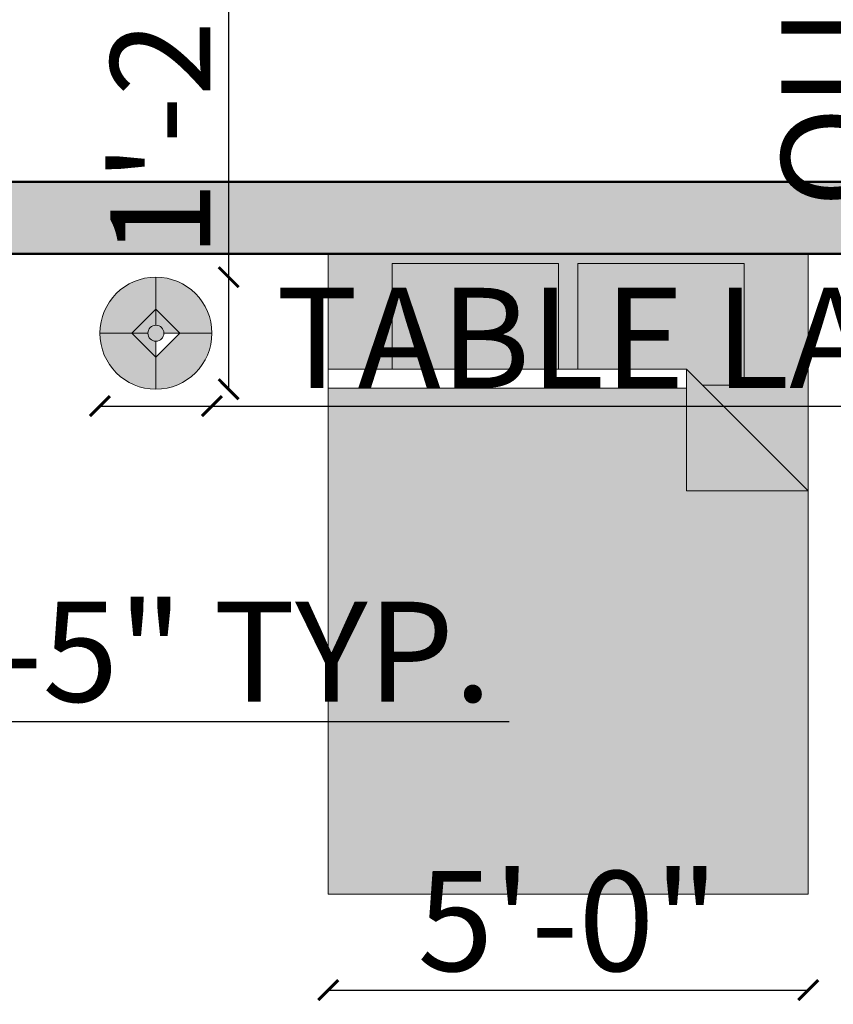
# Model space of a CAD drawing. Units: inches. Extents: x 2419 to 2878, y 1068 to 1713.
# Tile 17 of 20: x 2595 to 2697, y 1475 to 1598. Entities that reach past the tile are written whole.
import ezdxf

# ---------------------------------------------------------------- set-up
doc = ezdxf.new("R2010")
doc.units = ezdxf.units.IN
for name, color, linetype, lineweight in [('A-ANNO-DIMS', 2, 'Continuous', 18), ('A-FLOR-PRKG-PATT', 1, 'Continuous', 13), ('A-FURN', 8, 'Continuous', 18), ('A-FURN-PATT', 254, 'Continuous', 13), ('A-WALL', 7, 'Continuous', 50)]:
    doc.layers.add(name, color=color, linetype=linetype, lineweight=lineweight)
doc.layers.add('A-FLOR-FIXT-PATT', color=254, linetype='Continuous', lineweight=13, true_color=0xd7ebd2)
doc.layers.add('A-WALL-PATT', color=18, linetype='Continuous', lineweight=13, true_color=0x000000)
doc.styles.get("Standard").update_dxf_attribs({"font": 'arial.ttf'})
doc.dimstyles.new('ISO-25', dxfattribs={"dimtxt": 12.5, "dimasz": 2.5, "dimexe": 1.25, "dimexo": 0.625, "dimtad": 1, "dimdec": 0, "dimlunit": 4, "dimtxsty": 'Standard', "dimblk": 'ARCHTICK', "dimcen": 2.5, "dimse1": 1, "dimse2": 1, "dimclrd": 4, "dimadec": 0, "dimazin": 0, "dimtfac": 1, "dimtdec": 0, "dimtmove": 0, "dimatfit": 3, "dimfxl": 1, "dimarcsym": 0})

# ---------------------------------------------------------------- blocks, each defined once
blk = doc.blocks.new('Bed - Queen')
for p, q in [((0, -80.00003), (0, 0)), ((0, 0), (59.99999, 0)), ((59.99999, 0), (59.99999, -80.00003)), ((7.99999, -1.2), (28.79998, -1.2)), ((7.99999, -14.4), (7.99999, -1.2)), ((28.79998, -1.2), (28.79998, -14.4)), ((31.19999, -1.2), (51.99999, -1.2)), ((31.19999, -14.4), (31.19999, -1.2)), ((51.99999, -1.2), (51.99999, -16.4)), ((0, -14.4), (44.8, -14.4)), ((59.99999, -29.6), (44.8, -14.4)), ((44.8, -14.4), (44.8, -29.6)), ((44.8, -16.8), (0, -16.8)), ((51.99999, -16.4), (46.79936, -16.4)), ((44.8, -29.6), (59.99999, -29.6)), ((59.99999, -80.00003), (0, -80.00003))]:
    blk.add_line(p, q)
blk = doc.blocks.new('Lamp - Table')
for p, q in [((0, 7), (0, 1)), ((0, 3), (-3, 0)), ((3, 0), (0, 3)), ((-1, 0), (-7, 0)), ((-3, 0), (0, -3)), ((0, -3), (3, 0)), ((1, 0), (7, 0)), ((0, -1), (0, -7))]:
    blk.add_line(p, q)
for radius in [7, 1]:
    blk.add_circle((0, 0), radius)
blk = doc.blocks.new('_ArchTick')
at = {"color": 0, "linetype": 'ByBlock', "const_width": 0.15}
blk.add_lwpolyline([(-0.5, -0.5), (0.5, 0.5)], dxfattribs=at)
blk = doc.blocks.new('*D16')
at = {"layer": 'A-ANNO-DIMS', "color": 0, "lineweight": -2, "transparency": 16777216}
blk.add_line((2471.51, 1623.24), (2780.51, 1623.24), dxfattribs=at)
at = {"layer": 'Defpoints', "color": 0, "transparency": 16777216}
for p in [(2780.51, 1623.24), (2471.51, 1577.81), (2780.51, 1577.81)]:
    blk.add_point(p, dxfattribs=at)
at = {"layer": 'A-ANNO-DIMS', "color": 0, "lineweight": -2, "transparency": 16777216, "xscale": 2.5, "yscale": 2.5, "zscale": 2.5, "rotation": 180}
blk.add_blockref('_ArchTick', (2471.51, 1623.24), dxfattribs=at)
at = {"layer": 'A-ANNO-DIMS', "color": 0, "lineweight": -2, "transparency": 16777216, "xscale": 2.5, "yscale": 2.5, "zscale": 2.5}
blk.add_blockref('_ArchTick', (2780.51, 1623.24), dxfattribs=at)
at = {"layer": 'A-ANNO-DIMS', "color": 0, "transparency": 16777216, "insert": (2626.01, 1630.25), "char_height": 12.5, "attachment_point": 5}
blk.add_mtext('25\'-9"', dxfattribs=at)
blk = doc.blocks.new('*D22')
at = {"layer": 'A-ANNO-DIMS', "color": 4, "lineweight": -2, "transparency": 16777216}
for p, q in [((2513.7, 1510.38), (2530.82, 1510.38)), ((2530.82, 1510.38), (2656.31, 1510.38))]:
    blk.add_line(p, q, dxfattribs=at)
at = {"layer": 'Defpoints', "color": 0, "transparency": 16777216}
for p in [(2530.82, 1510.38), (2513.7, 1507.81), (2530.82, 1507.81)]:
    blk.add_point(p, dxfattribs=at)
at = {"layer": 'A-ANNO-DIMS', "color": 4, "lineweight": -2, "transparency": 16777216, "xscale": 2.5, "yscale": 2.5, "zscale": 2.5, "rotation": 180}
blk.add_blockref('_ArchTick', (2513.7, 1510.38), dxfattribs=at)
at = {"layer": 'A-ANNO-DIMS', "color": 4, "lineweight": -2, "transparency": 16777216, "xscale": 2.5, "yscale": 2.5, "zscale": 2.5}
blk.add_blockref('_ArchTick', (2530.82, 1510.38), dxfattribs=at)
at = {"layer": 'A-ANNO-DIMS', "color": 0, "transparency": 16777216, "insert": (2594.82, 1517.47), "char_height": 12.5, "attachment_point": 5}
blk.add_mtext('SINK 1\'-5" TYP.', dxfattribs=at)
blk = doc.blocks.new('*D24')
at = {"layer": 'A-ANNO-DIMS', "color": 4, "lineweight": -2, "transparency": 16777216}
for p, q in [((2605.13, 1549.79), (2619.13, 1549.79)), ((2619.13, 1549.79), (2811.96, 1549.79))]:
    blk.add_line(p, q, dxfattribs=at)
at = {"layer": 'Defpoints', "color": 0, "transparency": 16777216}
for p in [(2605.13, 1551.89), (2619.13, 1551.89), (2619.13, 1549.79)]:
    blk.add_point(p, dxfattribs=at)
at = {"layer": 'A-ANNO-DIMS', "color": 4, "lineweight": -2, "transparency": 16777216, "xscale": 2.5, "yscale": 2.5, "zscale": 2.5, "rotation": 180}
blk.add_blockref('_ArchTick', (2605.13, 1549.79), dxfattribs=at)
at = {"layer": 'A-ANNO-DIMS', "color": 4, "lineweight": -2, "transparency": 16777216, "xscale": 2.5, "yscale": 2.5, "zscale": 2.5}
blk.add_blockref('_ArchTick', (2619.13, 1549.79), dxfattribs=at)
at = {"layer": 'A-ANNO-DIMS', "color": 0, "transparency": 16777216, "insert": (2716.8, 1556.69), "char_height": 12.5, "attachment_point": 5}
blk.add_mtext('TABLE LAMP 1\'-2" TYP.', dxfattribs=at)
blk = doc.blocks.new('*D25')
at = {"layer": 'A-ANNO-DIMS', "color": 4, "lineweight": -2, "transparency": 16777216}
for p, q in [((2621.23, 1565.89), (2621.23, 1644.66)), ((2621.23, 1551.89), (2621.23, 1565.89))]:
    blk.add_line(p, q, dxfattribs=at)
at = {"layer": 'Defpoints', "color": 0, "transparency": 16777216}
for p in [(2619.13, 1565.89), (2621.23, 1565.89), (2619.13, 1551.89)]:
    blk.add_point(p, dxfattribs=at)
at = {"layer": 'A-ANNO-DIMS', "color": 4, "lineweight": -2, "transparency": 16777216, "xscale": 2.5, "yscale": 2.5, "zscale": 2.5}
for p, rotation in [((2621.23, 1565.89), 90), ((2621.23, 1551.89), 270)]:
    blk.add_blockref('_ArchTick', p, dxfattribs=dict(at, rotation=rotation))
at = {"layer": 'A-ANNO-DIMS', "color": 0, "transparency": 16777216, "insert": (2614.32, 1606.52), "char_height": 12.5, "attachment_point": 5, "rotation": 90}
blk.add_mtext('1\'-2" TYP.', dxfattribs=at)
blk = doc.blocks.new('*D30')
at = {"layer": 'A-ANNO-DIMS', "color": 4, "lineweight": -2, "transparency": 16777216}
for p, q in [((2705.68, 1568.81), (2705.68, 1713.47)), ((2705.68, 1488.81), (2705.68, 1568.81))]:
    blk.add_line(p, q, dxfattribs=at)
at = {"layer": 'Defpoints', "color": 0, "transparency": 16777216}
for p in [(2693.68, 1568.81), (2705.68, 1568.81), (2693.68, 1488.81)]:
    blk.add_point(p, dxfattribs=at)
at = {"layer": 'A-ANNO-DIMS', "color": 4, "lineweight": -2, "transparency": 16777216, "xscale": 2.5, "yscale": 2.5, "zscale": 2.5}
for p, rotation in [((2705.68, 1568.81), 90), ((2705.68, 1488.81), 270)]:
    blk.add_blockref('_ArchTick', p, dxfattribs=dict(at, rotation=rotation))
at = {"layer": 'A-ANNO-DIMS', "color": 0, "transparency": 16777216, "insert": (2698.21, 1642.39), "char_height": 12.5, "attachment_point": 5, "rotation": 90}
blk.add_mtext('QUEEN BED 6\'-8"', dxfattribs=at)
blk = doc.blocks.new('*D31')
at = {"layer": 'A-ANNO-DIMS', "color": 4, "lineweight": -2, "transparency": 16777216}
blk.add_line((2633.68, 1476.81), (2693.68, 1476.81), dxfattribs=at)
at = {"layer": 'Defpoints', "color": 0, "transparency": 16777216}
for p in [(2633.68, 1488.81), (2693.68, 1488.81), (2693.68, 1476.81)]:
    blk.add_point(p, dxfattribs=at)
at = {"layer": 'A-ANNO-DIMS', "color": 4, "lineweight": -2, "transparency": 16777216, "xscale": 2.5, "yscale": 2.5, "zscale": 2.5, "rotation": 180}
blk.add_blockref('_ArchTick', (2633.68, 1476.81), dxfattribs=at)
at = {"layer": 'A-ANNO-DIMS', "color": 4, "lineweight": -2, "transparency": 16777216, "xscale": 2.5, "yscale": 2.5, "zscale": 2.5}
blk.add_blockref('_ArchTick', (2693.68, 1476.81), dxfattribs=at)
at = {"layer": 'A-ANNO-DIMS', "color": 0, "transparency": 16777216, "insert": (2663.68, 1483.82), "char_height": 12.5, "attachment_point": 5}
blk.add_mtext('5\'-0"', dxfattribs=at)
blk = doc.blocks.new('*D36')
at = {"layer": 'A-ANNO-DIMS', "color": 4, "lineweight": -2, "transparency": 16777216}
blk.add_line((2656.74, 1605.01), (2736.32, 1605.01), dxfattribs=at)
at = {"layer": 'Defpoints', "color": 0, "transparency": 16777216}
for p in [(2736.32, 1605.01), (2656.74, 1205.81), (2736.32, 1205.81)]:
    blk.add_point(p, dxfattribs=at)
at = {"layer": 'A-ANNO-DIMS', "color": 4, "lineweight": -2, "transparency": 16777216, "xscale": 2.5, "yscale": 2.5, "zscale": 2.5, "rotation": 180}
blk.add_blockref('_ArchTick', (2656.74, 1605.01), dxfattribs=at)
at = {"layer": 'A-ANNO-DIMS', "color": 4, "lineweight": -2, "transparency": 16777216, "xscale": 2.5, "yscale": 2.5, "zscale": 2.5}
blk.add_blockref('_ArchTick', (2736.32, 1605.01), dxfattribs=at)
at = {"layer": 'A-ANNO-DIMS', "color": 0, "transparency": 16777216, "insert": (2696.53, 1612.1), "char_height": 12.5, "attachment_point": 5}
blk.add_mtext('6\'-7 1/2"', dxfattribs=at)
blk = doc.blocks.new('*D39')
at = {"layer": 'A-ANNO-DIMS', "color": 4, "lineweight": -2, "transparency": 16777216}
for p, q in [((2662.74, 1605.01), (2668.59, 1605.01)), ((2668.59, 1605.01), (2705.56, 1605.01))]:
    blk.add_line(p, q, dxfattribs=at)
at = {"layer": 'Defpoints', "color": 0, "transparency": 16777216}
for p in [(2668.59, 1605.01), (2662.74, 1165.6), (2668.59, 1165.6)]:
    blk.add_point(p, dxfattribs=at)
at = {"layer": 'A-ANNO-DIMS', "color": 4, "lineweight": -2, "transparency": 16777216, "xscale": 2.5, "yscale": 2.5, "zscale": 2.5, "rotation": 180}
blk.add_blockref('_ArchTick', (2662.74, 1605.01), dxfattribs=at)
at = {"layer": 'A-ANNO-DIMS', "color": 4, "lineweight": -2, "transparency": 16777216, "xscale": 2.5, "yscale": 2.5, "zscale": 2.5}
blk.add_blockref('_ArchTick', (2668.59, 1605.01), dxfattribs=at)
at = {"layer": 'A-ANNO-DIMS', "color": 0, "transparency": 16777216, "insert": (2688.32, 1612.02), "char_height": 12.5, "attachment_point": 5}
blk.add_mtext('0\'-6"', dxfattribs=at)
blk = doc.blocks.new('*D46')
at = {"layer": 'A-ANNO-DIMS', "color": 4, "lineweight": -2, "transparency": 16777216}
for p, q in [((2569.11, 1605.01), (2587.69, 1605.01)), ((2587.69, 1605.01), (2652.62, 1605.01))]:
    blk.add_line(p, q, dxfattribs=at)
at = {"layer": 'Defpoints', "color": 0, "transparency": 16777216}
for p in [(2587.69, 1605.01), (2569.11, 1512.81), (2587.69, 1512.81)]:
    blk.add_point(p, dxfattribs=at)
at = {"layer": 'A-ANNO-DIMS', "color": 4, "lineweight": -2, "transparency": 16777216, "xscale": 2.5, "yscale": 2.5, "zscale": 2.5, "rotation": 180}
blk.add_blockref('_ArchTick', (2569.11, 1605.01), dxfattribs=at)
at = {"layer": 'A-ANNO-DIMS', "color": 4, "lineweight": -2, "transparency": 16777216, "xscale": 2.5, "yscale": 2.5, "zscale": 2.5}
blk.add_blockref('_ArchTick', (2587.69, 1605.01), dxfattribs=at)
at = {"layer": 'A-ANNO-DIMS', "color": 0, "transparency": 16777216, "insert": (2621.41, 1612.1), "char_height": 12.5, "attachment_point": 5}
blk.add_mtext('1\'-6 1/2"', dxfattribs=at)
blk = doc.blocks.new('*D48')
at = {"layer": 'A-ANNO-DIMS', "color": 4, "lineweight": -2, "transparency": 16777216}
for p, q in [((2444.31, 1567.55), (2444.31, 1548.96)), ((2444.31, 1548.96), (2444.31, 1484.03))]:
    blk.add_line(p, q, dxfattribs=at)
at = {"layer": 'Defpoints', "color": 0, "transparency": 16777216}
for p in [(2725.51, 1567.55), (2444.31, 1548.96), (2725.51, 1548.96)]:
    blk.add_point(p, dxfattribs=at)
at = {"layer": 'A-ANNO-DIMS', "color": 4, "lineweight": -2, "transparency": 16777216, "xscale": 2.5, "yscale": 2.5, "zscale": 2.5}
for p, rotation in [((2444.31, 1567.55), 90), ((2444.31, 1548.96), 270)]:
    blk.add_blockref('_ArchTick', p, dxfattribs=dict(at, rotation=rotation))
at = {"layer": 'A-ANNO-DIMS', "color": 0, "transparency": 16777216, "insert": (2437.23, 1515.25), "char_height": 12.5, "attachment_point": 5, "rotation": 90}
blk.add_mtext('1\'-6 1/2"', dxfattribs=at)
blk = doc.blocks.new('*D50')
at = {"layer": 'A-ANNO-DIMS', "color": 4, "lineweight": -2, "transparency": 16777216}
for p, q in [((2444.31, 1458.39), (2444.31, 1494.19)), ((2444.31, 1437.39), (2444.31, 1458.39))]:
    blk.add_line(p, q, dxfattribs=at)
at = {"layer": 'Defpoints', "color": 0, "transparency": 16777216}
for p in [(2444.31, 1458.39), (2763.51, 1458.39), (2763.51, 1437.39)]:
    blk.add_point(p, dxfattribs=at)
at = {"layer": 'A-ANNO-DIMS', "color": 4, "lineweight": -2, "transparency": 16777216, "xscale": 2.5, "yscale": 2.5, "zscale": 2.5}
for p, rotation in [((2444.31, 1458.39), 90), ((2444.31, 1437.39), 270)]:
    blk.add_blockref('_ArchTick', p, dxfattribs=dict(at, rotation=rotation))
at = {"layer": 'A-ANNO-DIMS', "color": 0, "transparency": 16777216, "insert": (2437.31, 1477.54), "char_height": 12.5, "attachment_point": 5, "rotation": 90}
blk.add_mtext('1\'-9"', dxfattribs=at)
blk = doc.blocks.new('*D53')
at = {"layer": 'A-ANNO-DIMS', "color": 4, "lineweight": -2, "transparency": 16777216}
for p, q in [((2638.79, 1605.01), (2667.31, 1605.01)), ((2667.31, 1605.01), (2733.63, 1605.01))]:
    blk.add_line(p, q, dxfattribs=at)
at = {"layer": 'Defpoints', "color": 0, "transparency": 16777216}
for p in [(2667.31, 1605.01), (2638.79, 1217.38), (2667.31, 1217.38)]:
    blk.add_point(p, dxfattribs=at)
at = {"layer": 'A-ANNO-DIMS', "color": 4, "lineweight": -2, "transparency": 16777216, "xscale": 2.5, "yscale": 2.5, "zscale": 2.5, "rotation": 180}
blk.add_blockref('_ArchTick', (2638.79, 1605.01), dxfattribs=at)
at = {"layer": 'A-ANNO-DIMS', "color": 4, "lineweight": -2, "transparency": 16777216, "xscale": 2.5, "yscale": 2.5, "zscale": 2.5}
blk.add_blockref('_ArchTick', (2667.31, 1605.01), dxfattribs=at)
at = {"layer": 'A-ANNO-DIMS', "color": 0, "transparency": 16777216, "insert": (2701.72, 1612.1), "char_height": 12.5, "attachment_point": 5}
blk.add_mtext('2\'-4 1/2"', dxfattribs=at)

msp = doc.modelspace()

# ---------------------------------------------------------------- hatches: boundary and pattern name
at = {"layer": 'A-FLOR-FIXT-PATT'}
h = msp.add_hatch(color=256, dxfattribs=at)
h.dxf.hatch_style = 1
h.paths.add_polyline_path([(2705.38, 1406.81, 0.5), (2704.38, 1407.81), (2687.38, 1407.81, 0.5), (2686.38, 1406.81), (2686.38, 1402.81, 0.5), (2687.38, 1401.81), (2704.38, 1401.81, 0.5), (2705.38, 1402.81)])
h.paths.add_polyline_path([(2770.51, 1456.39, 0.5), (2769.51, 1457.39), (2765.51, 1457.39, 0.5), (2764.51, 1456.39), (2764.51, 1439.39, 0.5), (2765.51, 1438.39), (2769.51, 1438.39, 0.5), (2770.51, 1439.39)])
h.paths.add_polyline_path([(2641.68, 1567.61), (2662.48, 1567.61), (2662.48, 1554.41), (2664.88, 1554.41), (2664.88, 1567.61), (2685.68, 1567.61), (2685.68, 1552.41), (2680.48, 1552.41), (2693.68, 1539.21), (2693.68, 1568.81), (2633.68, 1568.81), (2633.68, 1554.41), (2641.68, 1554.41)])
h.paths.add_polyline_path([(2678.48, 1554.41), (2678.48, 1539.21), (2693.68, 1539.21)], flags=17)
h = msp.add_hatch(color=256, dxfattribs=at)
h.dxf.hatch_style = 1
h.paths.add_polyline_path([(2771.51, 1458.39), (2763.51, 1458.39), (2763.51, 1437.39), (2771.51, 1437.39)])
h.paths.add_polyline_path([(2770.51, 1456.39, 0.5), (2769.51, 1457.39), (2765.51, 1457.39, 0.5), (2764.51, 1456.39), (2764.51, 1439.39, 0.5), (2765.51, 1438.39), (2769.51, 1438.39, 0.5), (2770.51, 1439.39)], flags=16)
h.paths.add_polyline_path([(2706.38, 1408.81), (2685.38, 1408.81), (2685.38, 1400.81), (2706.38, 1400.81)])
h.paths.add_polyline_path([(2704.38, 1401.81, 0.5), (2705.38, 1402.81), (2705.38, 1406.81, 0.5), (2704.38, 1407.81), (2687.38, 1407.81, 0.5), (2686.38, 1406.81), (2686.38, 1402.81, 0.5), (2687.38, 1401.81)], flags=16)
h.paths.add_polyline_path([(2574.48, 1207.45), (2633.94, 1207.45), (2633.94, 1217.37), (2574.48, 1217.37)], flags=9)
h.paths.add_polyline_path([(2574.45, 1217.83), (2610.47, 1217.83), (2610.47, 1227.88), (2574.45, 1227.88)], flags=9)
h.paths.add_polyline_path([(2672.43, 1304.02), (2718.62, 1304.02), (2718.62, 1313.94), (2672.43, 1313.94)], flags=9)
h.paths.add_polyline_path([(2672.4, 1314.4), (2750.13, 1314.4), (2750.13, 1324.45), (2672.4, 1324.45)], flags=9)
h.paths.add_polyline_path([(2500.43, 1374.44), (2544.8, 1374.44), (2544.8, 1384.36), (2500.43, 1384.36)], flags=9)
h.paths.add_polyline_path([(2500.41, 1384.82), (2566.08, 1384.82), (2566.08, 1394.87), (2500.41, 1394.87)], flags=9)
h.paths.add_polyline_path([(2738.93, 1376.75), (2778.27, 1376.75), (2778.27, 1386.67), (2738.93, 1386.67)], flags=9)
h.paths.add_polyline_path([(2659.12, 1357.8), (2703.49, 1357.8), (2703.49, 1367.72), (2659.12, 1367.72)], flags=9)
h.paths.add_polyline_path([(2659.1, 1368.18), (2694.11, 1368.18), (2694.11, 1378.23), (2659.1, 1378.23)], flags=9)
h.paths.add_polyline_path([(2730.12, 1466.07), (2769.46, 1466.07), (2769.46, 1475.99), (2730.12, 1475.99)], flags=9)
h.paths.add_polyline_path([(2730.1, 1476.45), (2765.12, 1476.45), (2765.12, 1486.5), (2730.1, 1486.5)], flags=9)
h.paths.add_polyline_path([(2730.38, 1518.65), (2761.48, 1518.65), (2761.48, 1528.57), (2730.38, 1528.57)], flags=9)
h.paths.add_polyline_path([(2730.36, 1529.03), (2780.96, 1529.03), (2780.96, 1539.07), (2730.36, 1539.07)], flags=9)
h.paths.add_polyline_path([(2629.32, 1455.19), (2688.78, 1455.19), (2688.78, 1465.11), (2629.32, 1465.11)], flags=9)
h.paths.add_polyline_path([(2629.3, 1465.57), (2681.9, 1465.57), (2681.9, 1475.62), (2629.3, 1475.62)], flags=9)
h.paths.add_polyline_path([(2513.23, 1456.48), (2562.63, 1456.48), (2562.63, 1466.4), (2513.23, 1466.4)], flags=9)
h.paths.add_polyline_path([(2513.21, 1466.86), (2556.26, 1466.86), (2556.26, 1476.91), (2513.21, 1476.91)], flags=9)
h.paths.add_polyline_path([(2488.87, 1521.54), (2519.97, 1521.54), (2519.97, 1531.46), (2488.87, 1531.46)], flags=9)
h.paths.add_polyline_path([(2536.55, 1543.51), (2580.92, 1543.51), (2580.92, 1553.43), (2536.55, 1553.43)], flags=9)
h.paths.add_polyline_path([(2536.56, 1553.92), (2573.53, 1553.92), (2573.53, 1563.8), (2536.56, 1563.8)], flags=9)
at = {"layer": 'A-FLOR-PRKG-PATT'}
h = msp.add_hatch(color=256, dxfattribs=at)
h.dxf.hatch_style = 1
edge = h.paths.add_edge_path()
edge.add_ellipse((2561.37, 1279.45), major_axis=(3.99, 0), ratio=0.842304, start_angle=0.6466, end_angle=90)
edge.add_line((2561.37, 1282.81), (2511.57, 1282.81))
edge.add_ellipse((2511.57, 1279.45), major_axis=(3.99, 0), ratio=0.842304, start_angle=90, end_angle=179.3534)
edge.add_ellipse((10560.89, 1188.62), major_axis=(-8054.03, 0), ratio=0.8423039, start_angle=-0.646554, end_angle=-0.628237)
edge.add_ellipse((2509.23, 1276.91), major_axis=(1.69, 0), ratio=0.842304, start_angle=179.3718, end_angle=248.4648)
edge.add_ellipse((10560.33, 1188.62), major_axis=(8052.29, 0), ratio=0.8423039, start_angle=179.353446, end_angle=179.381357, ccw=False)
edge.add_ellipse((2511.01, 1279.45), major_axis=(2.25, 0), ratio=0.842304, start_angle=90, end_angle=179.3534, ccw=False)
edge.add_line((2511.01, 1281.35), (2561.94, 1281.35))
edge.add_ellipse((2561.94, 1279.45), major_axis=(-2.25, 0), ratio=0.842304, start_angle=180.6466, end_angle=270, ccw=False)
edge.add_ellipse((-5487.38, 1188.62), major_axis=(8052.29, 0), ratio=0.8423039, start_angle=0.528271, end_angle=0.646554, ccw=False)
edge.add_ellipse((2563.71, 1276.91), major_axis=(-1.69, 0), ratio=0.842304, start_angle=111.5352, end_angle=180.6282)
edge.add_ellipse((-5487.95, 1188.62), major_axis=(-8054.03, 0), ratio=0.8423039, start_angle=180.628237, end_angle=180.646554)
edge = h.paths.add_edge_path()
edge.add_ellipse((2564.91, 1261.91), major_axis=(-1.12, 0), ratio=0.842304, start_angle=180, end_angle=270)
edge.add_line((2564.91, 1262.86), (2564.43, 1262.86))
edge.add_ellipse((-5487.38, 1188.62), major_axis=(8052.29, 0), ratio=0.8423039, start_angle=0.383867, end_angle=0.528271, ccw=False)
edge.add_line((2564.65, 1242.56), (2564.91, 1242.56))
edge.add_ellipse((2564.91, 1243.51), major_axis=(-1.12, 0), ratio=0.842304, start_angle=90, end_angle=180)
edge.add_line((2566.03, 1243.51), (2566.03, 1261.91))
edge = h.paths.add_edge_path()
edge.add_ellipse((2564.91, 1174.99), major_axis=(1.12, 0), ratio=0.842304, start_angle=0, end_angle=90)
edge.add_line((2564.91, 1175.94), (2564.89, 1175.94))
edge.add_ellipse((-5487.38, 1188.62), major_axis=(8052.29, 0), ratio=0.8423039, start_angle=-0.134987, end_angle=-0.090229, ccw=False)
edge.add_ellipse((2163.34, 1170.91), major_axis=(401.54, 0), ratio=0.842304, start_angle=-2.18, end_angle=-0.1356, ccw=False)
edge.add_line((2564.47, 1155.64), (2564.91, 1155.64))
edge.add_ellipse((2564.91, 1156.59), major_axis=(-1.12, 0), ratio=0.842304, start_angle=90, end_angle=180)
edge.add_line((2566.03, 1156.59), (2566.03, 1174.99))
h.paths.add_polyline_path([(2574.48, 1207.45), (2633.94, 1207.45), (2633.94, 1217.37), (2574.48, 1217.37)], flags=9)
h.paths.add_polyline_path([(2574.45, 1217.83), (2610.47, 1217.83), (2610.47, 1227.88), (2574.45, 1227.88)], flags=9)
h.paths.add_polyline_path([(2672.43, 1304.02), (2718.62, 1304.02), (2718.62, 1313.94), (2672.43, 1313.94)], flags=9)
h.paths.add_polyline_path([(2672.4, 1314.4), (2750.13, 1314.4), (2750.13, 1324.45), (2672.4, 1324.45)], flags=9)
h.paths.add_polyline_path([(2500.43, 1374.44), (2544.8, 1374.44), (2544.8, 1384.36), (2500.43, 1384.36)], flags=9)
h.paths.add_polyline_path([(2500.41, 1384.82), (2566.08, 1384.82), (2566.08, 1394.87), (2500.41, 1394.87)], flags=9)
h.paths.add_polyline_path([(2738.93, 1376.75), (2778.27, 1376.75), (2778.27, 1386.67), (2738.93, 1386.67)], flags=9)
h.paths.add_polyline_path([(2659.12, 1357.8), (2703.49, 1357.8), (2703.49, 1367.72), (2659.12, 1367.72)], flags=9)
h.paths.add_polyline_path([(2659.1, 1368.18), (2694.11, 1368.18), (2694.11, 1378.23), (2659.1, 1378.23)], flags=9)
h.paths.add_polyline_path([(2730.12, 1466.07), (2769.46, 1466.07), (2769.46, 1475.99), (2730.12, 1475.99)], flags=9)
h.paths.add_polyline_path([(2730.1, 1476.45), (2765.12, 1476.45), (2765.12, 1486.5), (2730.1, 1486.5)], flags=9)
h.paths.add_polyline_path([(2730.38, 1518.65), (2761.48, 1518.65), (2761.48, 1528.57), (2730.38, 1528.57)], flags=9)
h.paths.add_polyline_path([(2730.36, 1529.03), (2780.96, 1529.03), (2780.96, 1539.07), (2730.36, 1539.07)], flags=9)
h.paths.add_polyline_path([(2629.32, 1455.19), (2688.78, 1455.19), (2688.78, 1465.11), (2629.32, 1465.11)], flags=9)
h.paths.add_polyline_path([(2629.3, 1465.57), (2681.9, 1465.57), (2681.9, 1475.62), (2629.3, 1475.62)], flags=9)
h.paths.add_polyline_path([(2513.23, 1456.48), (2562.63, 1456.48), (2562.63, 1466.4), (2513.23, 1466.4)], flags=9)
h.paths.add_polyline_path([(2513.21, 1466.86), (2556.26, 1466.86), (2556.26, 1476.91), (2513.21, 1476.91)], flags=9)
h.paths.add_polyline_path([(2488.87, 1521.54), (2519.97, 1521.54), (2519.97, 1531.46), (2488.87, 1531.46)], flags=9)
h.paths.add_polyline_path([(2536.55, 1543.51), (2580.92, 1543.51), (2580.92, 1553.43), (2536.55, 1553.43)], flags=9)
h.paths.add_polyline_path([(2536.56, 1553.92), (2573.53, 1553.92), (2573.53, 1563.8), (2536.56, 1563.8)], flags=9)
at = {"layer": 'A-FURN-PATT'}
h = msp.add_hatch(color=256, dxfattribs=at)
h.dxf.hatch_style = 1
h.paths.add_polyline_path([(2662.48, 1567.61), (2641.68, 1567.61), (2641.68, 1554.41), (2662.48, 1554.41)])
h.paths.add_polyline_path([(2685.68, 1567.61), (2664.88, 1567.61), (2664.88, 1554.41), (2678.48, 1554.41), (2680.48, 1552.41), (2685.68, 1552.41)])
h = msp.add_hatch(color=256, dxfattribs=at)
h.dxf.hatch_style = 1
h.paths.add_polyline_path([(2619.13, 1558.89), (2615.13, 1558.89), (2612.13, 1555.89), (2612.13, 1551.89, 0.414214)])
h.paths.add_polyline_path([(2612.13, 1565.89), (2612.13, 1561.89), (2615.13, 1558.89), (2619.13, 1558.89, 0.414214)])
h.paths.add_polyline_path([(2612.13, 1561.89), (2612.13, 1565.89, 0.414214), (2605.13, 1558.89), (2609.13, 1558.89)])
h.paths.add_polyline_path([(2612.13, 1555.89), (2609.13, 1558.89), (2605.13, 1558.89, 0.414214), (2612.13, 1551.89)])
h.paths.add_polyline_path([(2710.17, 1562.64), (2710.17, 1566.64, 0.414214), (2703.17, 1559.64), (2707.17, 1559.64)])
h.paths.add_polyline_path([(2710.17, 1556.64), (2707.17, 1559.64), (2703.17, 1559.64, 0.414214), (2710.17, 1552.64)])
h.paths.add_polyline_path([(2717.17, 1559.64), (2713.17, 1559.64), (2710.17, 1556.64), (2710.17, 1552.64, 0.414214)])
h.paths.add_polyline_path([(2710.17, 1566.64), (2710.17, 1562.64), (2713.17, 1559.64), (2717.17, 1559.64, 0.414214)])
h = msp.add_hatch(color=256, dxfattribs=at)
h.dxf.hatch_style = 1
h.paths.add_polyline_path([(2710.17, 1562.64), (2707.17, 1559.64), (2709.17, 1559.64, -0.414214), (2710.17, 1560.64)])
h.paths.add_polyline_path([(2711.17, 1559.64, 1), (2709.17, 1559.64, 1)])
h.paths.add_polyline_path([(2710.17, 1562.64), (2710.17, 1560.64, -0.414214), (2711.17, 1559.64), (2713.17, 1559.64)])
h.paths.add_polyline_path([(2713.17, 1559.64), (2711.17, 1559.64, -0.414214), (2710.17, 1558.64), (2710.17, 1556.64)])
h.paths.add_polyline_path([(2710.17, 1558.64, -0.414214), (2709.17, 1559.64), (2707.17, 1559.64), (2710.17, 1556.64)])
h.paths.add_polyline_path([(2613.13, 1558.89, 1), (2611.13, 1558.89, 1)])
h.paths.add_polyline_path([(2612.13, 1561.89), (2612.13, 1559.89, -0.414214), (2613.13, 1558.89), (2615.13, 1558.89)])
h.paths.add_polyline_path([(2612.13, 1559.89), (2612.13, 1561.89), (2609.13, 1558.89), (2611.13, 1558.89, -0.414214)])
h.paths.add_polyline_path([(2612.13, 1557.89, -0.414214), (2611.13, 1558.89), (2609.13, 1558.89), (2612.13, 1555.89)])
h.paths.add_polyline_path([(2574.48, 1207.45), (2633.94, 1207.45), (2633.94, 1217.37), (2574.48, 1217.37)], flags=9)
h.paths.add_polyline_path([(2574.45, 1217.83), (2610.47, 1217.83), (2610.47, 1227.88), (2574.45, 1227.88)], flags=9)
h.paths.add_polyline_path([(2672.43, 1304.02), (2718.62, 1304.02), (2718.62, 1313.94), (2672.43, 1313.94)], flags=9)
h.paths.add_polyline_path([(2672.4, 1314.4), (2750.13, 1314.4), (2750.13, 1324.45), (2672.4, 1324.45)], flags=9)
h.paths.add_polyline_path([(2500.43, 1374.44), (2544.8, 1374.44), (2544.8, 1384.36), (2500.43, 1384.36)], flags=9)
h.paths.add_polyline_path([(2500.41, 1384.82), (2566.08, 1384.82), (2566.08, 1394.87), (2500.41, 1394.87)], flags=9)
h.paths.add_polyline_path([(2738.93, 1376.75), (2778.27, 1376.75), (2778.27, 1386.67), (2738.93, 1386.67)], flags=9)
h.paths.add_polyline_path([(2659.12, 1357.8), (2703.49, 1357.8), (2703.49, 1367.72), (2659.12, 1367.72)], flags=9)
h.paths.add_polyline_path([(2659.1, 1368.18), (2694.11, 1368.18), (2694.11, 1378.23), (2659.1, 1378.23)], flags=9)
h.paths.add_polyline_path([(2730.12, 1466.07), (2769.46, 1466.07), (2769.46, 1475.99), (2730.12, 1475.99)], flags=9)
h.paths.add_polyline_path([(2730.1, 1476.45), (2765.12, 1476.45), (2765.12, 1486.5), (2730.1, 1486.5)], flags=9)
h.paths.add_polyline_path([(2730.38, 1518.65), (2761.48, 1518.65), (2761.48, 1528.57), (2730.38, 1528.57)], flags=9)
h.paths.add_polyline_path([(2730.36, 1529.03), (2780.96, 1529.03), (2780.96, 1539.07), (2730.36, 1539.07)], flags=9)
h.paths.add_polyline_path([(2629.32, 1455.19), (2688.78, 1455.19), (2688.78, 1465.11), (2629.32, 1465.11)], flags=9)
h.paths.add_polyline_path([(2629.3, 1465.57), (2681.9, 1465.57), (2681.9, 1475.62), (2629.3, 1475.62)], flags=9)
h.paths.add_polyline_path([(2513.23, 1456.48), (2562.63, 1456.48), (2562.63, 1466.4), (2513.23, 1466.4)], flags=9)
h.paths.add_polyline_path([(2513.21, 1466.86), (2556.26, 1466.86), (2556.26, 1476.91), (2513.21, 1476.91)], flags=9)
h.paths.add_polyline_path([(2488.87, 1521.54), (2519.97, 1521.54), (2519.97, 1531.46), (2488.87, 1531.46)], flags=9)
h.paths.add_polyline_path([(2536.55, 1543.51), (2580.92, 1543.51), (2580.92, 1553.43), (2536.55, 1553.43)], flags=9)
h.paths.add_polyline_path([(2536.56, 1553.92), (2573.53, 1553.92), (2573.53, 1563.8), (2536.56, 1563.8)], flags=9)
h = msp.add_hatch(color=256, dxfattribs=at)
h.dxf.hatch_style = 1
h.paths.add_polyline_path([(2693.68, 1539.21), (2678.48, 1539.21), (2678.48, 1552.01), (2633.68, 1552.01), (2633.68, 1488.81), (2693.68, 1488.81)])
edge = h.paths.add_edge_path()
edge.add_ellipse((2538.6, 1253.32), major_axis=(-60.49, 0), ratio=0.842304, start_angle=94.8701, end_angle=112.7919, ccw=False)
edge.add_line((2542.93, 1202.49), (2530.01, 1202.49))
edge.add_ellipse((2534.34, 1253.32), major_axis=(60.49, 0), ratio=0.842304, start_angle=247.2081, end_angle=265.1299, ccw=False)
edge.add_line((2514.16, 1205.28), (2512.5, 1192.83))
edge.add_ellipse((2532.38, 1242.44), major_axis=(-62.16, 0), ratio=0.842304, start_angle=68.165, end_angle=85.7226)
edge.add_line((2528.47, 1190.19), (2544.48, 1190.19))
edge.add_ellipse((2540.57, 1242.44), major_axis=(62.16, 0), ratio=0.842304, start_angle=-85.7226, end_angle=-68.165)
edge.add_line((2560.44, 1192.83), (2558.78, 1205.28))
edge = h.paths.add_edge_path()
edge.add_ellipse((2536.47, 1166.89), major_axis=(111.76, 0), ratio=0.842304, start_angle=76.4019, end_angle=103.5981)
edge.add_line((2514.16, 1259.13), (2514.16, 1244.82))
edge.add_ellipse((2536.47, 1152.59), major_axis=(111.76, 0), ratio=0.842304, start_angle=76.4019, end_angle=103.5981, ccw=False)
edge.add_line((2558.78, 1244.82), (2558.78, 1259.13))
at = {"layer": 'A-WALL-PATT'}
h = msp.add_hatch(color=256, dxfattribs=at)
h.dxf.hatch_style = 1
h.paths.add_polyline_path([(2780.51, 1577.81), (2471.51, 1577.81), (2471.51, 1121.81), (2780.51, 1121.81)])
h.paths.add_polyline_path([(2480.51, 1568.81), (2771.51, 1568.81), (2771.51, 1130.81), (2480.51, 1130.81)], flags=16)
h.paths.add_polyline_path([(2528.51, 1568.81), (2528.51, 1512.81), (2594.51, 1512.81), (2594.51, 1414.81), (2596.57, 1414.81), (2596.57, 1441.61), (2597.82, 1441.61), (2597.82, 1441.58, -0.384016), (2625.03, 1414.81), (2725.51, 1414.81), (2725.51, 1567.55), (2728.3, 1567.55), (2746.89, 1567.55), (2746.89, 1566.73), (2746.87, 1566.73, -0.367216), (2730.51, 1549.09), (2730.51, 1512.81), (2750.85, 1512.81), (2750.85, 1510.03, -0.401453), (2733.08, 1491.46), (2733.08, 1491.44), (2732.27, 1491.44), (2732.27, 1507.81), (2730.51, 1507.81), (2730.51, 1408.81), (2736.51, 1408.81), (2736.51, 1349.81), (2632.51, 1349.81), (2632.51, 1408.81), (2528.51, 1408.81), (2528.51, 1414.81), (2503.97, 1414.81), (2503.97, 1494.85), (2558.38, 1494.85), (2558.38, 1507.81), (2529.96, 1507.81, -0.414214), (2530.82, 1506.96), (2530.82, 1497.26, -0.414214), (2529.96, 1496.4), (2514.56, 1496.4, -0.414214), (2513.7, 1497.26), (2513.7, 1506.96, -0.414214), (2514.56, 1507.81), (2528.51, 1507.81), (2528.51, 1512.81), (2480.51, 1512.81)], flags=0)
h.paths.add_polyline_path([(2516.26, 1507.81), (2528.26, 1507.81), (2528.26, 1505.81), (2523.42, 1505.81), (2524.07, 1504.67), (2529.39, 1504.67, -0.414214), (2529.96, 1504.1), (2529.96, 1497.83, -0.414214), (2529.39, 1497.26), (2515.13, 1497.26, -0.414214), (2514.56, 1497.83), (2514.56, 1504.1, -0.414214), (2515.13, 1504.67), (2520.69, 1504.67), (2521.34, 1505.81), (2516.26, 1505.81)], flags=0)
h.paths.add_polyline_path([(2522.02, 1505.53), (2522.82, 1507.32, -0.65506), (2522.25, 1506.06), (2522.19, 1505.93), (2522.43, 1505.53)], flags=0)
h.paths.add_polyline_path([(2522.83, 1500.97, -1), (2521.69, 1500.97, -1)], flags=0)
h.paths.add_polyline_path([(2522.55, 1500.97, -1), (2521.98, 1500.97, -1)], flags=0)
h.paths.add_polyline_path([(2482.01, 1470.63), (2499.89, 1470.63), (2499.89, 1448.27), (2482.01, 1448.27), (2482.01, 1452.74), (2481.26, 1452.74), (2481.26, 1449.76), (2480.51, 1449.76), (2480.51, 1469.14), (2481.26, 1469.14), (2481.26, 1466.16), (2482.01, 1466.16)], flags=0)
h.paths.add_polyline_path([(2488.71, 1466.16, -1), (2484.24, 1466.16, -1)], flags=0)
h.paths.add_polyline_path([(2496.17, 1466.16, -1), (2490.2, 1466.16, -1)], flags=0)
h.paths.add_polyline_path([(2487.97, 1466.16, -1), (2484.99, 1466.16, -1)], flags=0)
h.paths.add_polyline_path([(2495.42, 1466.16, -1), (2490.95, 1466.16, -1)], flags=0)
h.paths.add_polyline_path([(2487.22, 1466.16, -1), (2485.73, 1466.16, -1)], flags=0)
h.paths.add_polyline_path([(2494.68, 1466.16, -1), (2491.69, 1466.16, -1)], flags=0)
h.paths.add_polyline_path([(2499.11, 1468, -1), (2497.98, 1468, -1)], flags=0)
h.paths.add_polyline_path([(2493.93, 1466.16, -1), (2492.44, 1466.16, -1)], flags=0)
h.paths.add_polyline_path([(2499.37, 1463.71, -1), (2498.17, 1463.71, -1)], flags=0)
h.paths.add_polyline_path([(2484.24, 1461.69), (2496.17, 1461.69), (2496.17, 1457.22), (2484.24, 1457.22)], flags=0)
h.paths.add_polyline_path([(2484.99, 1460.94), (2495.42, 1460.94), (2495.42, 1457.96), (2484.99, 1457.96)], flags=0)
h.paths.add_polyline_path([(2586.88, 1510.03), (2587.69, 1510.03), (2587.69, 1491.44), (2586.88, 1491.44)], flags=0)
h.paths.add_polyline_path([(2499.26, 1459.41, -1), (2498.2, 1459.41, -1)], flags=0)
h.paths.add_polyline_path([(2489.46, 1452.74, -1), (2483.5, 1452.74, -1)], flags=0)
h.paths.add_polyline_path([(2557.3, 1408.81), (2557.3, 1413.09, -0.401453), (2584.57, 1441.58), (2584.57, 1441.61), (2585.82, 1441.61), (2585.82, 1413.09), (2585.82, 1408.81)], flags=0)
h.paths.add_polyline_path([(2488.71, 1452.74, -1), (2484.24, 1452.74, -1)], flags=0)
h.paths.add_polyline_path([(2495.42, 1452.74, -1), (2490.95, 1452.74, -1)], flags=0)
h.paths.add_polyline_path([(2487.97, 1452.74, -1), (2484.99, 1452.74, -1)], flags=0)
h.paths.add_polyline_path([(2494.68, 1452.74, -1), (2491.69, 1452.74, -1)], flags=0)
h.paths.add_polyline_path([(2487.22, 1452.74, -1), (2485.73, 1452.74, -1)], flags=0)
h.paths.add_polyline_path([(2499.18, 1454.44, -1), (2497.9, 1454.44, -1)], flags=0)
h.paths.add_polyline_path([(2493.93, 1452.74, -1), (2492.44, 1452.74, -1)], flags=0)
h.paths.add_polyline_path([(2499.3, 1450.64, -1), (2497.79, 1450.64, -1)], flags=0)
h.paths.add_polyline_path([(2619.13, 1558.89, -1), (2605.13, 1558.89, -1)], flags=0)
h.paths.add_polyline_path([(2609.13, 1558.89), (2612.13, 1561.89), (2615.13, 1558.89), (2612.13, 1555.89)], flags=0)
h.paths.add_polyline_path([(2611.13, 1558.89, -1), (2613.13, 1558.89, -1)], flags=0)
h.paths.add_polyline_path([(2633.68, 1568.81), (2693.68, 1568.81), (2693.68, 1488.81), (2633.68, 1488.81)], flags=0)
h.paths.add_polyline_path([(2641.68, 1554.41), (2641.68, 1567.61), (2662.48, 1567.61), (2662.48, 1554.41), (2664.88, 1554.41), (2664.88, 1567.61), (2685.68, 1567.61), (2685.68, 1552.41), (2680.48, 1552.41), (2693.68, 1539.21), (2678.48, 1539.21), (2678.48, 1554.41)], flags=0)
h.paths.add_polyline_path([(2637.51, 1408.81), (2731.51, 1408.81), (2731.51, 1354.81), (2637.51, 1354.81), (2637.51, 1357.98), (2635.3, 1357.98), (2635.3, 1358.79), (2637.51, 1358.79)], flags=0)
h.paths.add_polyline_path([(2717.17, 1559.64, -1), (2703.17, 1559.64, -1)], flags=0)
h.paths.add_polyline_path([(2707.17, 1559.64), (2710.17, 1562.64), (2713.17, 1559.64), (2710.17, 1556.64)], flags=0)
h.paths.add_polyline_path([(2709.17, 1559.64, -1), (2711.17, 1559.64, -1)], flags=0)
h.paths.add_polyline_path([(2685.38, 1408.81), (2706.38, 1408.81), (2706.38, 1400.81), (2699.88, 1400.81), (2701.88, 1394.81, -0.501323), (2696.92, 1375.95, -0.132891), (2694.83, 1375.95, -0.501317), (2689.88, 1394.81), (2691.88, 1400.81), (2688.88, 1400.81), (2688.88, 1399.31), (2685.88, 1399.31), (2685.88, 1400.31), (2687.88, 1400.31), (2687.88, 1400.81), (2685.38, 1400.81)], flags=0)
h.paths.add_polyline_path([(2687.38, 1407.81), (2704.38, 1407.81, -0.5), (2705.38, 1406.81), (2705.38, 1402.81, -0.5), (2704.38, 1401.81), (2687.38, 1401.81, -0.5), (2686.38, 1402.81), (2686.38, 1406.81, -0.5)], flags=0)
h.paths.add_polyline_path([(2639.51, 1205.81), (2634.51, 1205.81), (2634.51, 1293.81), (2637.51, 1293.81), (2639.51, 1293.81)], flags=0)
h.paths.add_polyline_path([(2691.88, 1394.81), (2699.88, 1394.81, -0.48008), (2697.52, 1377.29, -0.215004), (2694.23, 1377.29, -0.48008)], flags=0)
h.paths.add_polyline_path([(2757.51, 1453.89), (2763.51, 1451.89), (2763.51, 1454.89), (2762.01, 1454.89), (2762.01, 1457.89), (2763.01, 1457.89), (2763.01, 1455.89), (2763.51, 1455.89), (2763.51, 1458.39), (2771.51, 1458.39), (2771.51, 1437.39), (2763.51, 1437.39), (2763.51, 1443.89), (2757.51, 1441.89, -0.501323), (2738.65, 1446.85, -0.132891), (2738.65, 1448.94, -0.501317)], flags=0)
h.paths.add_polyline_path([(2739.99, 1449.54, -0.48008), (2757.51, 1451.89), (2757.51, 1443.89, -0.48008), (2739.99, 1446.25, -0.215004)], flags=0)
h.paths.add_polyline_path([(2765.51, 1457.39), (2769.51, 1457.39, -0.5), (2770.51, 1456.39), (2770.51, 1439.39, -0.5), (2769.51, 1438.39), (2765.51, 1438.39, -0.5), (2764.51, 1439.39), (2764.51, 1456.39, -0.5)], flags=0)
h = msp.add_hatch(color=256, dxfattribs=at)
h.dxf.hatch_style = 1
h.paths.add_polyline_path([(2771.51, 1354.81), (2736.51, 1354.81), (2736.51, 1408.81), (2771.51, 1408.81), (2771.51, 1414.81), (2625.03, 1414.81, -0.015108), (2625.09, 1413.09), (2625.09, 1408.81), (2632.51, 1408.81), (2632.51, 1376.56), (2635.3, 1376.56, -0.029838), (2637.51, 1376.43), (2637.51, 1408.81), (2731.51, 1408.81), (2731.51, 1354.81), (2637.51, 1354.81), (2637.51, 1357.98), (2635.3, 1357.98), (2632.51, 1357.98), (2632.51, 1349.81), (2771.51, 1349.81)])
h.paths.add_polyline_path([(2639.51, 1298.81), (2637.51, 1298.81), (2480.51, 1298.81), (2480.51, 1293.81), (2637.51, 1293.81), (2639.51, 1293.81)])
h.paths.add_polyline_path([(2639.51, 1293.81), (2637.51, 1293.81), (2634.51, 1293.81), (2634.51, 1244.65), (2638.79, 1244.65, -0.006332), (2639.51, 1244.64)])
h.paths.add_polyline_path([(2639.51, 1205.81), (2771.51, 1205.81), (2771.51, 1210.81), (2639.51, 1210.81), (2639.51, 1216.13), (2638.79, 1216.13), (2634.51, 1216.13), (2634.51, 1130.81), (2639.51, 1130.81)])
h.paths.add_polyline_path([(2596.57, 1413.09), (2596.57, 1414.81), (2585.82, 1414.81), (2585.82, 1413.09), (2585.82, 1408.81), (2596.57, 1408.81)])
h.paths.add_polyline_path([(2557.3, 1413.09, -0.015108), (2557.35, 1414.81), (2480.51, 1414.81), (2480.51, 1408.81), (2557.3, 1408.81)])
h.paths.add_polyline_path([(2574.48, 1207.45), (2633.94, 1207.45), (2633.94, 1217.37), (2574.48, 1217.37)], flags=9)
h.paths.add_polyline_path([(2574.45, 1217.83), (2610.47, 1217.83), (2610.47, 1227.88), (2574.45, 1227.88)], flags=9)
h.paths.add_polyline_path([(2672.43, 1304.02), (2718.62, 1304.02), (2718.62, 1313.94), (2672.43, 1313.94)], flags=9)
h.paths.add_polyline_path([(2672.4, 1314.4), (2750.13, 1314.4), (2750.13, 1324.45), (2672.4, 1324.45)], flags=9)
h.paths.add_polyline_path([(2500.43, 1374.44), (2544.8, 1374.44), (2544.8, 1384.36), (2500.43, 1384.36)], flags=9)
h.paths.add_polyline_path([(2500.41, 1384.82), (2566.08, 1384.82), (2566.08, 1394.87), (2500.41, 1394.87)], flags=9)
h.paths.add_polyline_path([(2738.93, 1376.75), (2778.27, 1376.75), (2778.27, 1386.67), (2738.93, 1386.67)], flags=9)
h.paths.add_polyline_path([(2659.12, 1357.8), (2703.49, 1357.8), (2703.49, 1367.72), (2659.12, 1367.72)], flags=25)
h.paths.add_polyline_path([(2659.1, 1368.18), (2694.11, 1368.18), (2694.11, 1378.23), (2659.1, 1378.23)], flags=25)
h.paths.add_polyline_path([(2730.12, 1466.07), (2769.46, 1466.07), (2769.46, 1475.99), (2730.12, 1475.99)], flags=9)
h.paths.add_polyline_path([(2730.1, 1476.45), (2765.12, 1476.45), (2765.12, 1486.5), (2730.1, 1486.5)], flags=9)
h.paths.add_polyline_path([(2730.38, 1518.65), (2761.48, 1518.65), (2761.48, 1528.57), (2730.38, 1528.57)], flags=9)
h.paths.add_polyline_path([(2730.36, 1529.03), (2780.96, 1529.03), (2780.96, 1539.07), (2730.36, 1539.07)], flags=9)
h.paths.add_polyline_path([(2629.32, 1455.19), (2688.78, 1455.19), (2688.78, 1465.11), (2629.32, 1465.11)], flags=9)
h.paths.add_polyline_path([(2629.3, 1465.57), (2681.9, 1465.57), (2681.9, 1475.62), (2629.3, 1475.62)], flags=9)
h.paths.add_polyline_path([(2513.23, 1456.48), (2562.63, 1456.48), (2562.63, 1466.4), (2513.23, 1466.4)], flags=9)
h.paths.add_polyline_path([(2513.21, 1466.86), (2556.26, 1466.86), (2556.26, 1476.91), (2513.21, 1476.91)], flags=9)
h.paths.add_polyline_path([(2488.87, 1521.54), (2519.97, 1521.54), (2519.97, 1531.46), (2488.87, 1531.46)], flags=9)
h.paths.add_polyline_path([(2536.55, 1543.51), (2580.92, 1543.51), (2580.92, 1553.43), (2536.55, 1553.43)], flags=9)
h.paths.add_polyline_path([(2536.56, 1553.92), (2573.53, 1553.92), (2573.53, 1563.8), (2536.56, 1563.8)], flags=9)

# ---------------------------------------------------------------- linework, layer by layer
at = {"layer": 'A-WALL'}
msp.add_line((2480.51, 1568.81), (2771.51, 1568.81), dxfattribs=at)
msp.add_lwpolyline([(2471.51, 1577.81), (2780.51, 1577.81), (2780.51, 1121.81), (2471.51, 1121.81)], close=True, dxfattribs=at)

# ---------------------------------------------------------------- block references
at = {"layer": 'A-FURN'}
for name, p in [('Bed - Queen', (2633.68, 1568.81)), ('Lamp - Table', (2612.13, 1558.89))]:
    msp.add_blockref(name, p, dxfattribs=at)

# ---------------------------------------------------------------- dimensions: what is measured, and where the dimension line sits
at = {"layer": 'A-ANNO-DIMS'}
for base, p1, p2, text, picture, middle in [((2705.68, 1568.81), (2693.68, 1488.81), (2693.68, 1568.81), 'QUEEN BED <>', '*D30', (2698.21, 1642.39)), ((2621.23, 1565.89), (2619.13, 1551.89), (2619.13, 1565.89), '<> TYP.', '*D25', (2614.32, 1606.52))]:
    dim = msp.add_linear_dim(base=base, p1=p1, p2=p2, angle=90, text=text, dimstyle='ISO-25', override={"dimdec": 1, "dimlfac": 1, "dimrnd": 0, "dimzin": 1, "dimdsep": 46, "dimlunit": 4, "dimfrac": 2}, dxfattribs=at)
    dim.commit()
    dim.dimension.update_dxf_attribs({"geometry": picture, "text_midpoint": middle})
for base, p1, p2, override, picture, middle in [((2780.51, 1623.24), (2471.51, 1577.81), (2780.51, 1577.81), {"dimclrd": 0, "dimclre": 0, "dimclrt": 0}, '*D16', (2626.01, 1630.25)), ((2587.69, 1605.01), (2569.11, 1512.81), (2587.69, 1512.81), {"dimdec": 1, "dimlfac": 1, "dimrnd": 0, "dimzin": 1, "dimdsep": 46, "dimlunit": 4, "dimfrac": 2}, '*D46', (2621.41, 1612.1)), ((2667.31, 1605.01), (2638.79, 1217.38), (2667.31, 1217.38), {"dimdec": 1, "dimlfac": 1, "dimrnd": 0, "dimzin": 1, "dimdsep": 46, "dimlunit": 4, "dimfrac": 2}, '*D53', (2701.72, 1612.1)), ((2736.32, 1605.01), (2656.74, 1205.81), (2736.32, 1205.81), {"dimdec": 1, "dimlfac": 1, "dimrnd": 0, "dimzin": 1, "dimdsep": 46, "dimlunit": 4, "dimfrac": 2}, '*D36', (2696.53, 1612.1)), ((2668.5856, 1605.013), (2662.7408, 1165.6026), (2668.5856, 1165.6026), {"dimdec": 1, "dimlfac": 1, "dimrnd": 0, "dimzin": 1, "dimdsep": 46, "dimlunit": 4, "dimfrac": 2}, '*D39', (2688.3247, 1612.0201)), ((2693.68, 1476.81), (2633.68, 1488.81), (2693.68, 1488.81), {"dimdec": 1, "dimlfac": 1, "dimrnd": 0, "dimzin": 1, "dimdsep": 46, "dimlunit": 4, "dimfrac": 2}, '*D31', (2663.68, 1483.82))]:
    dim = msp.add_linear_dim(base=base, p1=p1, p2=p2, dimstyle='ISO-25', override=override, dxfattribs=at)
    dim.commit()
    dim.dimension.update_dxf_attribs({"geometry": picture, "text_midpoint": middle})
for base, p1, p2, text, picture, middle in [((2619.13, 1549.79), (2605.13, 1551.89), (2619.13, 1551.89), 'TABLE LAMP <> TYP.', '*D24', (2716.8, 1556.69)), ((2530.82, 1510.38), (2513.7, 1507.81), (2530.82, 1507.81), 'SINK <> TYP.', '*D22', (2594.82, 1517.47))]:
    dim = msp.add_linear_dim(base=base, p1=p1, p2=p2, text=text, dimstyle='ISO-25', override={"dimdec": 1, "dimlfac": 1, "dimrnd": 0, "dimzin": 1, "dimdsep": 46, "dimlunit": 4, "dimfrac": 2}, dxfattribs=at)
    dim.commit()
    dim.dimension.update_dxf_attribs({"geometry": picture, "text_midpoint": middle})
for base, p1, p2, picture, middle in [((2444.31, 1548.96), (2725.51, 1567.55), (2725.51, 1548.96), '*D48', (2437.23, 1515.25)), ((2444.31, 1458.39), (2763.51, 1437.39), (2763.51, 1458.39), '*D50', (2437.31, 1477.54))]:
    dim = msp.add_linear_dim(base=base, p1=p1, p2=p2, angle=90, dimstyle='ISO-25', override={"dimdec": 1, "dimlfac": 1, "dimrnd": 0, "dimzin": 1, "dimdsep": 46, "dimlunit": 4, "dimfrac": 2}, dxfattribs=at)
    dim.commit()
    dim.dimension.update_dxf_attribs({"geometry": picture, "text_midpoint": middle})

doc.saveas('drawing.dxf')
